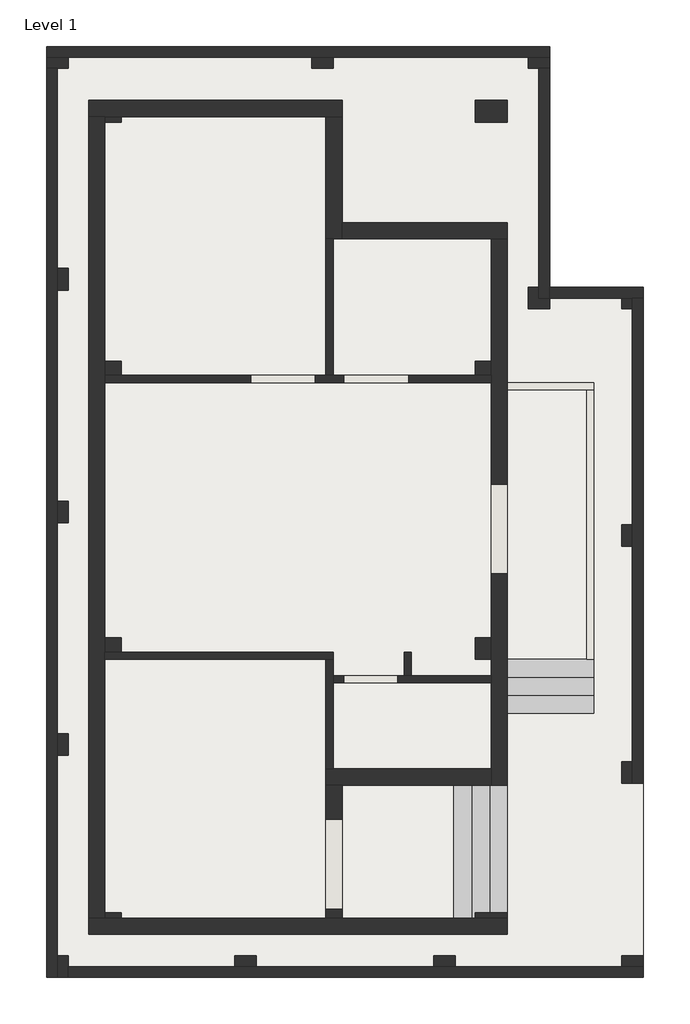
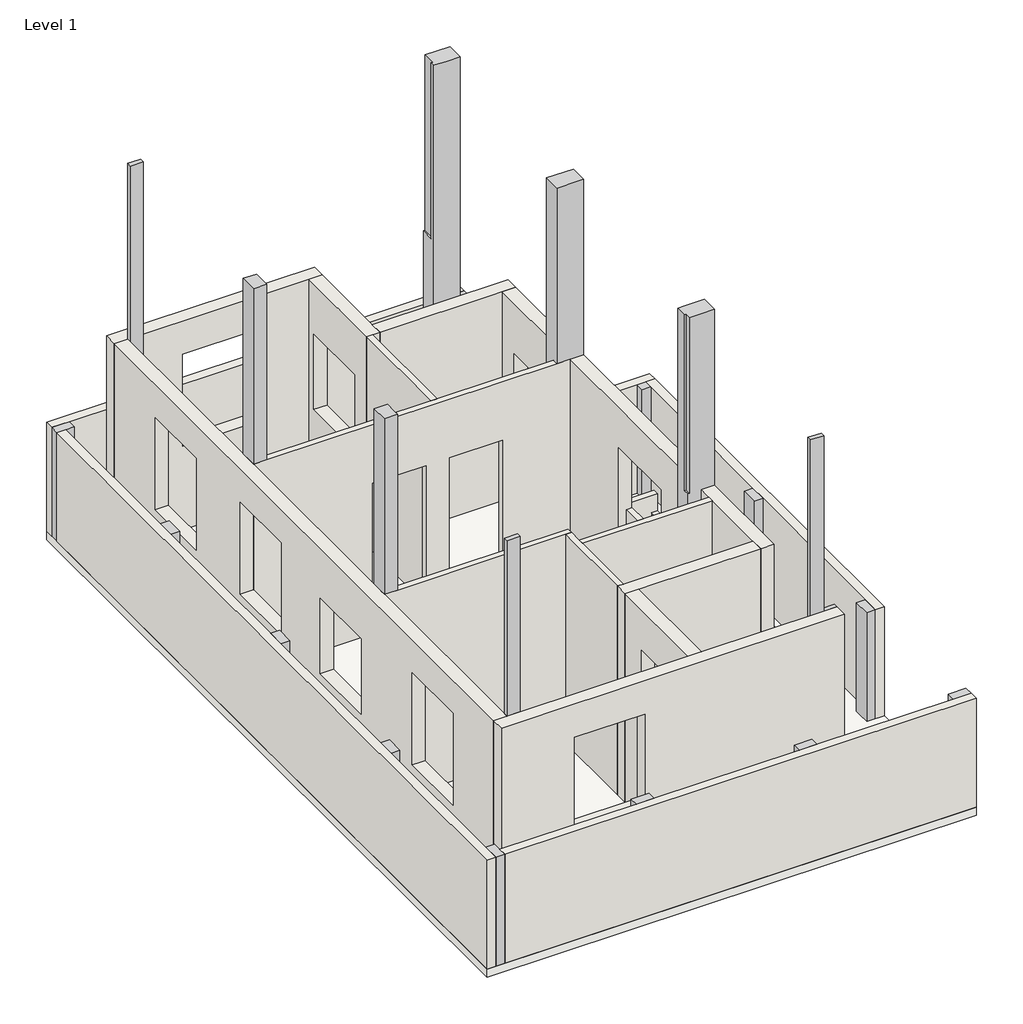
# One storey: 22 columns, 22 walls, 2 stair flights, 1 slab.
"""IFC4 building model written with IfcOpenShell, lengths in millimetres."""

from ifc_helpers import new_model, si_unit, frame, origin, origin_with_axes, place, context, project, spatial, polyline, outline, extrude, faceted_brep, element, save

model = new_model("IFC4")

# Units and contexts
model_context = context("Model", 3, world=origin())
ifc_project = project(units=[si_unit("LENGTHUNIT", "METRE", prefix="MILLI")], contexts=[model_context])

# Site, building, storey
site = spatial("IfcSite", under=ifc_project)
building = spatial("IfcBuilding", under=site)
storey = spatial("IfcBuildingStorey", under=building, Name="Level 1", Elevation=0.0)

# Columns
placement = place(None, origin())
element("IfcColumn", 1, ObjectType="Rectangular Column : 1'6\" x 1'", at=placement, inside=storey, context=model_context, shape_type="Brep", body=[
    faceted_brep([(398.6834347, -3882.8142443, 0.0), (855.8834347, -3882.8142443, 0.0), (855.8834347, -3959.0142443, 0.0), (398.6834347, -3959.0142443, 0.0), (398.6834347, -3882.8142443, 7010.4), (627.2834347, -3882.8142443, 7010.4), (627.2834347, -3882.8142443, 3810.0), (855.8834347, -3882.8142443, 3810.0), (855.8834347, -3959.0142443, 3810.0), (398.6834347, -3959.0142443, 3810.0), (398.6834347, -3959.0142443, 7010.4), (627.2834347, -3959.0142443, 7010.4), (627.2834347, -3959.0142443, 3810.0)], [[[0, 1, 2, 3]], [[1, 0, 4, 5, 6, 7]], [[2, 1, 7, 8]], [[4, 0, 3, 9, 10]], [[4, 10, 11, 5]], [[3, 2, 8, 12, 9]], [[10, 9, 12, 11]], [[12, 6, 5, 11]], [[6, 12, 8, 7]]]),
])
element("IfcColumn", 2, ObjectType="Rectangular Column : 1'6\" x 1'", at=placement, inside=storey, context=model_context, shape_type="Brep", body=[
    faceted_brep([(-4605.1165653, -3882.8142443, 0.0), (-4605.1165653, -3959.0142443, 0.0), (-4833.7165653, -3959.0142443, 0.0), (-4833.7165653, -3882.8142443, 0.0), (-4605.1165653, -3882.8142443, 7010.4), (-4833.7165653, -3882.8142443, 3810.0), (-4833.7165653, -3882.8142443, 7010.4), (-4605.1165653, -3959.0142443, 7010.4), (-4605.1165653, -3959.0142443, 3810.0), (-4833.7165653, -3959.0142443, 7010.4), (-4833.7165653, -3959.0142443, 3810.0)], [[[0, 1, 2, 3]], [[4, 0, 3, 5, 6]], [[0, 4, 7, 8, 1]], [[4, 6, 9, 7]], [[1, 8, 10, 2]], [[3, 2, 10, 5]], [[6, 5, 10, 9]], [[8, 7, 9, 10]]]),
])
element("IfcColumn", 3, ObjectType="Rectangular Column : 1'6\" x 1'", at=placement, inside=storey, context=model_context, shape_type="Brep", body=[
    faceted_brep([(-4833.7165653, 3.3857557, 0.0), (-4605.1165653, 3.3857557, 0.0), (-4605.1165653, -199.8142443, 0.0), (-4833.7165653, -199.8142443, 0.0), (-4605.1165653, 3.3857557, 7010.4), (-4833.7165653, 3.3857557, 1524.0), (-4833.7165653, 3.3857557, 2895.6), (-4833.7165653, 3.3857557, 3810.0), (-4833.7165653, 3.3857557, 7010.4), (-4605.1165653, -199.8142443, 7010.4), (-4605.1165653, -301.4142443, 7010.4), (-4605.1165653, -301.4142443, 3810.0), (-4605.1165653, -199.8142443, 3810.0), (-4833.7165653, -301.4142443, 7010.4), (-4833.7165653, -301.4142443, 3810.0), (-4833.7165653, -199.8142443, 3810.0)], [[[0, 1, 2, 3]], [[4, 1, 0, 5, 6, 7, 8]], [[1, 4, 9, 10, 11, 12, 2]], [[11, 10, 13, 14]], [[10, 9, 4, 8, 13]], [[5, 0, 3, 15, 7, 6]], [[12, 15, 3, 2]], [[15, 12, 11, 14]], [[8, 7, 15, 14, 13]]]),
])
element("IfcColumn", 4, ObjectType="Rectangular Column : 1'6\" x 1'", at=placement, inside=storey, context=model_context, shape_type="Brep", body=[
    faceted_brep([(398.6834347, -301.4142443, 0.0), (398.6834347, 3.3857557, 0.0), (627.2834347, 3.3857557, 0.0), (627.2834347, -301.4142443, 0.0), (398.6834347, 3.3857557, 7010.4), (525.6834347, 3.3857557, 7010.4), (627.2834347, 3.3857557, 7010.4), (855.8834347, 3.3857557, 7010.4), (855.8834347, 3.3857557, 3810.0), (627.2834347, 3.3857557, 3810.0), (855.8834347, -301.4142443, 7010.4), (855.8834347, -301.4142443, 3810.0), (627.2834347, -301.4142443, 3810.0), (627.2834347, -301.4142443, 7010.4), (424.0834347, -301.4142443, 7010.4), (424.0834347, -301.4142443, 3810.0), (398.6834347, -301.4142443, 3810.0), (398.6834347, -199.8142443, 3810.0), (398.6834347, -199.8142443, 7010.4), (424.0834347, -199.8142443, 7010.4), (424.0834347, -199.8142443, 3810.0)], [[[0, 1, 2, 3]], [[4, 5, 6, 7, 8, 9, 2, 1]], [[7, 10, 11, 8]], [[0, 3, 12, 11, 10, 13, 14, 15, 16]], [[1, 0, 16, 17, 18, 4]], [[7, 6, 5, 4, 18, 19, 14, 13, 10]], [[3, 2, 9, 12]], [[12, 9, 8, 11]], [[20, 19, 18, 17]], [[15, 20, 17, 16]], [[19, 20, 15, 14]]]),
])
element("IfcColumn", 5, ObjectType="Rectangular Column : 1'6\" x 1'", at=placement, inside=storey, context=model_context, shape_type="Brep", body=[
    faceted_brep([(398.6834347, 3914.9857557, 0.0), (627.2834347, 3914.9857557, 0.0), (627.2834347, 3711.7857557, 0.0), (398.6834347, 3711.7857557, 0.0), (398.6834347, 3914.9857557, 7010.4), (855.8834347, 3914.9857557, 7010.4), (855.8834347, 3914.9857557, 3810.0), (627.2834347, 3914.9857557, 3810.0), (855.8834347, 3610.1857557, 7010.4), (855.8834347, 3610.1857557, 3810.0), (627.2834347, 3610.1857557, 7010.4), (525.6834347, 3610.1857557, 7010.4), (398.6834347, 3610.1857557, 7010.4), (398.6834347, 3610.1857557, 6096.0), (398.6834347, 3610.1857557, 4724.4), (398.6834347, 3610.1857557, 3810.0), (525.6834347, 3610.1857557, 3810.0), (627.2834347, 3610.1857557, 3810.0), (398.6834347, 3711.7857557, 3810.0), (398.6834347, 3711.7857557, 7010.4), (627.2834347, 3711.7857557, 3810.0)], [[[0, 1, 2, 3]], [[4, 5, 6, 7, 1, 0]], [[5, 8, 9, 6]], [[8, 10, 11, 12, 13, 14, 15, 16, 17, 9]], [[4, 0, 3, 18, 15, 14, 13, 12, 19]], [[5, 4, 19, 12, 11, 10, 8]], [[1, 7, 20, 2]], [[7, 6, 9, 17, 20]], [[20, 18, 3, 2]], [[18, 20, 17, 16, 15]]]),
])
element("IfcColumn", 6, ObjectType="Rectangular Column : 1'6\" x 1'", at=placement, inside=storey, context=model_context, shape_type="Brep", body=[
    faceted_brep([(-4833.7165653, 3914.9857557, 0.0), (-4605.1165653, 3914.9857557, 0.0), (-4605.1165653, 3711.7857557, 0.0), (-4833.7165653, 3711.7857557, 0.0), (-4605.1165653, 3914.9857557, 7010.4), (-4833.7165653, 3914.9857557, 3810.0), (-4833.7165653, 3914.9857557, 7010.4), (-4605.1165653, 3711.7857557, 7010.4), (-4605.1165653, 3610.1857557, 7010.4), (-4605.1165653, 3610.1857557, 3810.0), (-4605.1165653, 3711.7857557, 3810.0), (-4833.7165653, 3610.1857557, 7010.4), (-4833.7165653, 3610.1857557, 3810.0), (-4833.7165653, 3711.7857557, 3810.0)], [[[0, 1, 2, 3]], [[4, 1, 0, 5, 6]], [[1, 4, 7, 8, 9, 10, 2]], [[9, 8, 11, 12]], [[8, 7, 4, 6, 11]], [[5, 0, 3, 13]], [[10, 13, 3, 2]], [[13, 10, 9, 12]], [[6, 5, 13, 12, 11]]]),
])
element("IfcColumn", 7, ObjectType="Rectangular Column : 1'6\" x 1'", at=placement, inside=storey, context=model_context, shape_type="Brep", body=[
    faceted_brep([(-4605.1165653, 7369.3857557, 0.0), (-4605.1165653, 7293.1857557, 0.0), (-4833.7165653, 7293.1857557, 0.0), (-4833.7165653, 7369.3857557, 0.0), (-4605.1165653, 7293.1857557, 7010.4), (-4605.1165653, 7369.3857557, 3810.0), (-4605.1165653, 7369.3857557, 7010.4), (-4833.7165653, 7293.1857557, 7010.4), (-4833.7165653, 7293.1857557, 3810.0), (-4833.7165653, 7369.3857557, 7010.4), (-4833.7165653, 7369.3857557, 3810.0)], [[[0, 1, 2, 3]], [[4, 1, 0, 5, 6]], [[1, 4, 7, 8, 2]], [[4, 6, 9, 7]], [[5, 0, 3, 10]], [[3, 2, 8, 10]], [[6, 5, 10, 9]], [[8, 7, 9, 10]]]),
])
element("IfcColumn", 8, ObjectType="Rectangular Column : 1'6\" x 1'", at=placement, inside=storey, context=model_context, shape_type="Brep", body=[
    faceted_brep([(398.6834347, 7597.9857557, 0.0), (855.8834347, 7597.9857557, 0.0), (855.8834347, 7293.1857557, 0.0), (398.6834347, 7293.1857557, 0.0), (398.6834347, 7597.9857557, 3810.0), (424.0834347, 7597.9857557, 3810.0), (424.0834347, 7597.9857557, 7010.4), (855.8834347, 7597.9857557, 7010.4), (855.8834347, 7293.1857557, 7010.4), (855.8834347, 7293.1857557, 3810.0), (627.2834347, 7293.1857557, 7010.4), (398.6834347, 7293.1857557, 7010.4), (398.6834347, 7369.3857557, 7010.4), (398.6834347, 7369.3857557, 3810.0), (424.0834347, 7369.3857557, 7010.4), (424.0834347, 7369.3857557, 3810.0)], [[[0, 1, 2, 3]], [[1, 0, 4, 5, 6, 7]], [[2, 1, 7, 8, 9]], [[3, 2, 9, 8, 10, 11]], [[0, 3, 11, 12, 13, 4]], [[8, 7, 6, 14, 12, 11, 10]], [[14, 15, 13, 12]], [[15, 5, 4, 13]], [[15, 14, 6, 5]]]),
])
element("IfcColumn", 9, ObjectType="Rectangular Column : 1'x1'", at=placement, inside=storey, context=model_context, shape_type="SweptSolid", body=[
    extrude(outline(polyline([(-5354.4165653, 5223.0857557), (-5354.4165653, 4918.2857557), (-5506.8165653, 4918.2857557), (-5506.8165653, 5223.0857557), (-5354.4165653, 5223.0857557)])), origin_with_axes(), (0.0, 0.0, 1.0), 1981.2),
])
element("IfcColumn", 10, ObjectType="Rectangular Column : 1'x1'", at=placement, inside=storey, context=model_context, shape_type="Brep", body=[
    faceted_brep([(-5354.4165653, 8055.1857557, 0.0), (-5506.8165653, 8055.1857557, 0.0), (-5659.2165653, 8055.1857557, 0.0), (-5659.2165653, 8207.5857557, 0.0), (-5354.4165653, 8207.5857557, 0.0), (-5354.4165653, 8055.1857557, 1981.2), (-5354.4165653, 8207.5857557, 1981.2), (-5506.8165653, 8055.1857557, 1981.2), (-5659.2165653, 8055.1857557, 1981.2), (-5659.2165653, 8207.5857557, 1981.2)], [[[0, 1, 2, 3, 4]], [[5, 0, 4, 6]], [[2, 1, 0, 5, 7, 8]], [[2, 8, 9, 3]], [[8, 7, 5, 6, 9]], [[4, 3, 9, 6]]]),
])
element("IfcColumn", 11, ObjectType="Rectangular Column : 1'x1'", at=placement, inside=storey, context=model_context, shape_type="SweptSolid", body=[
    extrude(outline(polyline([(-1607.9165653, 8055.1857557), (-1912.7165653, 8055.1857557), (-1912.7165653, 8207.5857557), (-1607.9165653, 8207.5857557), (-1607.9165653, 8055.1857557)])), origin_with_axes(), (0.0, 0.0, 1.0), 1981.2),
])
element("IfcColumn", 12, ObjectType="Rectangular Column : 1'x1'", at=placement, inside=storey, context=model_context, shape_type="Brep", body=[
    faceted_brep([(1452.7834347, 8055.1857557, 0.0), (1300.3834347, 8055.1857557, 0.0), (1147.9834347, 8055.1857557, 0.0), (1147.9834347, 8207.5857557, 0.0), (1452.7834347, 8207.5857557, 0.0), (1452.7834347, 8055.1857557, 1981.2), (1452.7834347, 8207.5857557, 1981.2), (1300.3834347, 8055.1857557, 1981.2), (1147.9834347, 8055.1857557, 1981.2), (1147.9834347, 8207.5857557, 1981.2)], [[[0, 1, 2, 3, 4]], [[5, 0, 4, 6]], [[2, 1, 0, 5, 7, 8]], [[2, 8, 9, 3]], [[8, 7, 5, 6, 9]], [[4, 3, 9, 6]]]),
])
element("IfcColumn", 13, ObjectType="Rectangular Column : 1'x1'", at=placement, inside=storey, context=model_context, shape_type="SweptSolid", body=[
    extrude(outline(polyline([(1452.7834347, 4651.5857557), (1147.9834347, 4651.5857557), (1147.9834347, 4956.3857557), (1300.3834347, 4956.3857557), (1300.3834347, 4803.9857557), (1452.7834347, 4803.9857557), (1452.7834347, 4651.5857557)])), origin_with_axes(), (0.0, 0.0, 1.0), 1981.2),
])
element("IfcColumn", 14, ObjectType="Rectangular Column : 1'x1'", at=placement, inside=storey, context=model_context, shape_type="SweptSolid", body=[
    extrude(outline(polyline([(2468.7834347, 4651.5857557), (2468.7834347, 4803.9857557), (2621.1834347, 4803.9857557), (2621.1834347, 4651.5857557), (2468.7834347, 4651.5857557)])), origin_with_axes(), (0.0, 0.0, 1.0), 1981.2),
])
element("IfcColumn", 15, ObjectType="Rectangular Column : 1'x1'", at=placement, inside=storey, context=model_context, shape_type="SweptSolid", body=[
    extrude(outline(polyline([(-5354.4165653, 1933.7857557), (-5354.4165653, 1628.9857557), (-5506.8165653, 1628.9857557), (-5506.8165653, 1933.7857557), (-5354.4165653, 1933.7857557)])), origin_with_axes(), (0.0, 0.0, 1.0), 1981.2),
])
element("IfcColumn", 16, ObjectType="Rectangular Column : 1'x1'", at=placement, inside=storey, context=model_context, shape_type="SweptSolid", body=[
    extrude(outline(polyline([(-5354.4165653, -1355.5142443), (-5354.4165653, -1660.3142443), (-5506.8165653, -1660.3142443), (-5506.8165653, -1355.5142443), (-5354.4165653, -1355.5142443)])), origin_with_axes(), (0.0, 0.0, 1.0), 1981.2),
])
element("IfcColumn", 17, ObjectType="Rectangular Column : 1'x1'", at=placement, inside=storey, context=model_context, shape_type="Brep", body=[
    faceted_brep([(-5354.4165653, -4492.4142443, 0.0), (-5354.4165653, -4644.8142443, 0.0), (-5354.4165653, -4797.2142443, 0.0), (-5506.8165653, -4797.2142443, 0.0), (-5506.8165653, -4492.4142443, 0.0), (-5354.4165653, -4492.4142443, 1981.2), (-5354.4165653, -4644.8142443, 1981.2), (-5354.4165653, -4797.2142443, 1981.2), (-5506.8165653, -4797.2142443, 1981.2), (-5506.8165653, -4492.4142443, 1981.2)], [[[0, 1, 2, 3, 4]], [[2, 1, 0, 5, 6, 7]], [[2, 7, 8, 3]], [[5, 0, 4, 9]], [[7, 6, 5, 9, 8]], [[4, 3, 8, 9]]]),
])
element("IfcColumn", 18, ObjectType="Rectangular Column : 1'x1'", at=placement, inside=storey, context=model_context, shape_type="SweptSolid", body=[
    extrude(outline(polyline([(-3000.683232, -4492.4142443), (-2695.883232, -4492.4142443), (-2695.883232, -4644.8142443), (-3000.683232, -4644.8142443), (-3000.683232, -4492.4142443)])), origin_with_axes(), (0.0, 0.0, 1.0), 1981.2),
])
element("IfcColumn", 19, ObjectType="Rectangular Column : 1'x1'", at=placement, inside=storey, context=model_context, shape_type="SweptSolid", body=[
    extrude(outline(polyline([(-189.7498986, -4492.4142443), (115.0501014, -4492.4142443), (115.0501014, -4644.8142443), (-189.7498986, -4644.8142443), (-189.7498986, -4492.4142443)])), origin_with_axes(), (0.0, 0.0, 1.0), 1981.2),
])
element("IfcColumn", 20, ObjectType="Rectangular Column : 1'x1'", at=placement, inside=storey, context=model_context, shape_type="SweptSolid", body=[
    extrude(outline(polyline([(2468.7834347, -4492.4142443), (2773.5834347, -4492.4142443), (2773.5834347, -4644.8142443), (2468.7834347, -4644.8142443), (2468.7834347, -4492.4142443)])), origin_with_axes(), (0.0, 0.0, 1.0), 1981.2),
])
element("IfcColumn", 21, ObjectType="Rectangular Column : 1'x1'", at=placement, inside=storey, context=model_context, shape_type="SweptSolid", body=[
    extrude(outline(polyline([(2468.7834347, -2054.0142443), (2468.7834347, -1749.2142443), (2621.1834347, -1749.2142443), (2621.1834347, -2054.0142443), (2468.7834347, -2054.0142443)])), origin_with_axes(), (0.0, 0.0, 1.0), 1981.2),
])
element("IfcColumn", 22, ObjectType="Rectangular Column : 1'x1'", at=placement, inside=storey, context=model_context, shape_type="SweptSolid", body=[
    extrude(outline(polyline([(2468.7834347, 1298.7857557), (2468.7834347, 1603.5857557), (2621.1834347, 1603.5857557), (2621.1834347, 1298.7857557), (2468.7834347, 1298.7857557)])), origin_with_axes(), (0.0, 0.0, 1.0), 1981.2),
])

# Slab
element("IfcSlab", 23, ObjectType="6\" floor", at=placement, inside=storey, context=model_context, shape_type="SweptSolid", body=[
    extrude(outline(polyline([(-5659.2165653, 8359.9857557), (1452.7834347, 8359.9857557), (1452.7834347, 4956.3857557), (2773.5834347, 4956.3857557), (2773.5834347, -4797.2142443), (-5659.2165653, -4797.2142443), (-5659.2165653, 8359.9857557)])), frame((0.0, 0.0, -152.4), z_axis=(0.0, 0.0, 1.0), x_axis=(1.0, 0.0, 0.0)), (0.0, 0.0, 1.0), 152.4),
])

# Stair flights
element("IfcStairFlight", 24, ObjectType="3/4\" Nosing", at=placement, inside=storey, context=model_context, shape_type="Brep", body=[
    faceted_brep([(855.8834347, -2079.4142443, 152.4), (855.8834347, -3882.8142443, 152.4), (836.8334347, -3882.8142443, 0.0), (836.8334347, -2079.4142443, 0.0), (582.8334347, -2079.4142443, 152.4), (582.8334347, -3882.8142443, 152.4), (582.8334347, -3882.8142443, 0.0), (582.8334347, -2079.4142443, 0.0), (347.8834347, -3959.0142443, 457.2), (347.8834347, -2079.4142443, 457.2), (93.8834347, -2079.4142443, 457.2), (93.8834347, -3959.0142443, 457.2), (328.8334347, -3959.0142443, 0.0), (328.8334347, -3959.0142443, 304.8), (93.8834347, -3959.0142443, 0.0), (328.8334347, -2079.4142443, 304.8), (328.8334347, -2079.4142443, 0.0), (93.8834347, -2079.4142443, 0.0), (398.6834347, -3882.8142443, 0.0), (398.6834347, -3959.0142443, 0.0), (398.6834347, -3959.0142443, 304.8), (398.6834347, -3882.8142443, 304.8), (601.8834347, -3882.8142443, 304.8), (601.8834347, -2079.4142443, 304.8)], [[[0, 1, 2, 3]], [[1, 0, 4, 5]], [[1, 5, 6, 2]], [[4, 0, 3, 7]], [[8, 9, 10, 11]], [[12, 13, 8, 11, 14]], [[15, 16, 17, 10, 9]], [[11, 10, 17, 14]], [[13, 15, 9, 8]], [[2, 6, 18, 19, 12, 14, 17, 16, 7, 3]], [[13, 20, 21, 22, 23, 15]], [[20, 13, 12, 19]], [[21, 20, 19, 18]], [[6, 5, 22, 21, 18]], [[4, 7, 16, 15, 23]], [[5, 4, 23, 22]]]),
])
element("IfcStairFlight", 25, ObjectType="3/4\" Nosing", at=placement, inside=storey, context=model_context, shape_type="Brep", body=[
    faceted_brep([(2075.0834347, -1063.4142443, 152.4), (855.8834347, -1063.4142443, 152.4), (855.8834347, -1044.3642443, 0.0), (2075.0834347, -1044.3642443, 0.0), (2075.0834347, -790.3642443, 152.4), (855.8834347, -790.3642443, 152.4), (855.8834347, -790.3642443, 0.0), (2075.0834347, -790.3642443, 0.0), (855.8834347, -809.4142443, 304.8), (2075.0834347, -809.4142443, 304.8), (2075.0834347, -536.3642443, 304.8), (855.8834347, -536.3642443, 304.8), (855.8834347, -536.3642443, 0.0), (2075.0834347, -536.3642443, 0.0), (855.8834347, -555.4142443, 457.2), (2075.0834347, -555.4142443, 457.2), (2075.0834347, -301.4142443, 457.2), (855.8834347, -301.4142443, 457.2), (855.8834347, -301.4142443, 0.0), (2075.0834347, -301.4142443, 0.0)], [[[0, 1, 2, 3]], [[1, 0, 4, 5]], [[1, 5, 6, 2]], [[4, 0, 3, 7]], [[8, 9, 10, 11]], [[6, 5, 8, 11, 12]], [[4, 7, 13, 10, 9]], [[5, 4, 9, 8]], [[14, 15, 16, 17]], [[12, 11, 14, 17, 18]], [[10, 13, 19, 16, 15]], [[17, 16, 19, 18]], [[11, 10, 15, 14]], [[2, 6, 12, 18, 19, 13, 7, 3]]]),
])

# Walls
element("IfcWall", 26, at=placement, inside=storey, context=model_context, shape_type="Brep", body=[
    faceted_brep([(-4833.7165653, 3610.1857557, 0.0), (627.2834347, 3610.1857557, 0.0), (627.2834347, 3610.1857557, 3810.0), (398.6834347, 3610.1857557, 3810.0), (-4605.1165653, 3610.1857557, 3810.0), (-4833.7165653, 3610.1857557, 3810.0), (-4833.7165653, 3610.1857557, 3200.4), (-4833.7165653, 3610.1857557, 1524.0), (-2776.3165653, 3610.1857557, 609.6), (-2776.3165653, 3610.1857557, 2743.2), (-1861.9165653, 3610.1857557, 2743.2), (-1861.9165653, 3610.1857557, 609.6), (-541.1165653, 3610.1857557, 609.6), (-1455.5165653, 3610.1857557, 609.6), (-1455.5165653, 3610.1857557, 2743.2), (-541.1165653, 3610.1857557, 2743.2), (-4833.7165653, 3711.7857557, 0.0), (-4833.7165653, 3711.7857557, 3810.0), (-4605.1165653, 3711.7857557, 3810.0), (-1709.5165653, 3711.7857557, 3810.0), (-1607.9165653, 3711.7857557, 3810.0), (398.6834347, 3711.7857557, 3810.0), (627.2834347, 3711.7857557, 3810.0), (627.2834347, 3711.7857557, 0.0), (398.6834347, 3711.7857557, 0.0), (-1607.9165653, 3711.7857557, 0.0), (-1709.5165653, 3711.7857557, 0.0), (-4605.1165653, 3711.7857557, 0.0), (-2776.3165653, 3711.7857557, 609.6), (-1861.9165653, 3711.7857557, 609.6), (-1861.9165653, 3711.7857557, 2743.2), (-2776.3165653, 3711.7857557, 2743.2), (-541.1165653, 3711.7857557, 609.6), (-541.1165653, 3711.7857557, 2743.2), (-1455.5165653, 3711.7857557, 2743.2), (-1455.5165653, 3711.7857557, 609.6)], [[[0, 1, 2, 3, 4, 5, 6, 7], [8, 9, 10, 11], [12, 13, 14, 15]], [[16, 17, 18, 19, 20, 21, 22, 23, 24, 25, 26, 27], [28, 29, 30, 31], [32, 33, 34, 35]], [[1, 0, 16, 27, 26, 25, 24, 23]], [[5, 4, 3, 2, 22, 21, 20, 19, 18, 17]], [[0, 7, 6, 5, 17, 16]], [[2, 1, 23, 22]], [[29, 28, 8, 11]], [[30, 29, 11, 10]], [[31, 30, 10, 9]], [[28, 31, 9, 8]], [[13, 12, 32, 35]], [[14, 13, 35, 34]], [[15, 14, 34, 33]], [[12, 15, 33, 32]]]),
])
element("IfcWall", 27, at=placement, inside=storey, context=model_context, shape_type="SweptSolid", body=[
    extrude(outline(polyline([(-1709.5165653, 3711.7857557), (-1709.5165653, 5642.1857557), (-1607.9165653, 5642.1857557), (-1607.9165653, 3711.7857557), (-1709.5165653, 3711.7857557)])), origin_with_axes(), (0.0, 0.0, 1.0), 3810.0),
])
element("IfcWall", 28, at=placement, inside=storey, context=model_context, shape_type="Brep", body=[
    faceted_brep([(-4833.7165653, -301.4142443, 0.0), (-1709.5165653, -301.4142443, 0.0), (-1607.9165653, -301.4142443, 0.0), (-1607.9165653, -301.4142443, 3810.0), (-1709.5165653, -301.4142443, 3810.0), (-4605.1165653, -301.4142443, 3810.0), (-4833.7165653, -301.4142443, 3810.0), (-4833.7165653, -199.8142443, 0.0), (-4833.7165653, -199.8142443, 3810.0), (-4605.1165653, -199.8142443, 3810.0), (-1607.9165653, -199.8142443, 3810.0), (-1607.9165653, -199.8142443, 0.0), (-4605.1165653, -199.8142443, 0.0)], [[[0, 1, 2, 3, 4, 5, 6]], [[7, 8, 9, 10, 11, 12]], [[2, 1, 0, 7, 12, 11]], [[6, 5, 4, 3, 10, 9, 8]], [[0, 6, 8, 7]], [[3, 2, 11, 10]]]),
])
element("IfcWall", 29, at=placement, inside=storey, context=model_context, shape_type="Brep", body=[
    faceted_brep([(-1709.5165653, -301.4142443, 0.0), (-1709.5165653, -1850.8142443, 0.0), (-1709.5165653, -1850.8142443, 3810.0), (-1709.5165653, -301.4142443, 3810.0), (-1607.9165653, -301.4142443, 0.0), (-1607.9165653, -301.4142443, 3810.0), (-1607.9165653, -530.0142443, 3810.0), (-1607.9165653, -631.6142443, 3810.0), (-1607.9165653, -1850.8142443, 3810.0), (-1607.9165653, -1850.8142443, 0.0), (-1607.9165653, -631.6142443, 0.0), (-1607.9165653, -530.0142443, 0.0)], [[[0, 1, 2, 3]], [[4, 5, 6, 7, 8, 9, 10, 11]], [[1, 0, 4, 11, 10, 9]], [[3, 2, 8, 7, 6, 5]], [[0, 3, 5, 4]], [[2, 1, 9, 8]]]),
])
element("IfcWall", 30, at=placement, inside=storey, context=model_context, shape_type="Brep", body=[
    faceted_brep([(627.2834347, -530.0142443, 0.0), (-503.6379361, -530.0142443, 0.0), (-605.2379361, -530.0142443, 0.0), (-1607.9165653, -530.0142443, 0.0), (-1607.9165653, -530.0142443, 3810.0), (-605.2379361, -530.0142443, 3810.0), (-503.6379361, -530.0142443, 3810.0), (627.2834347, -530.0142443, 3810.0), (-693.5165653, -530.0142443, 609.6), (-693.5165653, -530.0142443, 2743.2), (-1455.5165653, -530.0142443, 2743.2), (-1455.5165653, -530.0142443, 609.6), (627.2834347, -631.6142443, 0.0), (627.2834347, -631.6142443, 3810.0), (-1607.9165653, -631.6142443, 3810.0), (-1607.9165653, -631.6142443, 0.0), (-693.5165653, -631.6142443, 609.6), (-1455.5165653, -631.6142443, 609.6), (-1455.5165653, -631.6142443, 2743.2), (-693.5165653, -631.6142443, 2743.2)], [[[0, 1, 2, 3, 4, 5, 6, 7], [8, 9, 10, 11]], [[12, 13, 14, 15], [16, 17, 18, 19]], [[3, 2, 1, 0, 12, 15]], [[7, 6, 5, 4, 14, 13]], [[0, 7, 13, 12]], [[4, 3, 15, 14]], [[17, 16, 8, 11]], [[18, 17, 11, 10]], [[19, 18, 10, 9]], [[16, 19, 9, 8]]]),
])
element("IfcWall", 31, at=placement, inside=storey, context=model_context, shape_type="SweptSolid", body=[
    extrude(outline(polyline([(-503.6379361, -199.8142443), (-503.6379361, -530.0142443), (-605.2379361, -530.0142443), (-605.2379361, -199.8142443), (-503.6379361, -199.8142443)])), origin_with_axes(), (0.0, 0.0, 1.0), 3810.0),
])
element("IfcWall", 32, at=placement, inside=storey, context=model_context, shape_type="Brep", body=[
    faceted_brep([(855.8834347, 3508.5857557, 0.0), (1973.4834347, 3508.5857557, 0.0), (2075.0834347, 3508.5857557, 0.0), (2075.0834347, 3508.5857557, 609.6), (2075.0834347, 3508.5857557, 914.4), (855.8834347, 3508.5857557, 914.4), (855.8834347, 3610.1857557, 0.0), (855.8834347, 3610.1857557, 914.4), (2075.0834347, 3610.1857557, 914.4), (2075.0834347, 3610.1857557, 0.0)], [[[0, 1, 2, 3, 4, 5]], [[6, 7, 8, 9]], [[2, 1, 0, 6, 9]], [[5, 4, 8, 7]], [[0, 5, 7, 6]], [[4, 3, 2, 9, 8]]]),
])
element("IfcWall", 33, at=placement, inside=storey, context=model_context, shape_type="SweptSolid", body=[
    extrude(outline(polyline([(1973.4834347, -301.4142443), (1973.4834347, 3508.5857557), (2075.0834347, 3508.5857557), (2075.0834347, -301.4142443), (1973.4834347, -301.4142443)])), origin_with_axes(), (0.0, 0.0, 1.0), 609.6),
])
element("IfcWall", 34, ObjectType="6\" wall", at=placement, inside=storey, context=model_context, shape_type="Brep", body=[
    faceted_brep([(-5659.2165653, 8055.1857557, 0.0), (-5659.2165653, -4797.2142443, 0.0), (-5659.2165653, -4797.2142443, 1981.2), (-5659.2165653, 8055.1857557, 1981.2), (-5506.8165653, 8055.1857557, 0.0), (-5506.8165653, 8055.1857557, 1981.2), (-5506.8165653, 5223.0857557, 1981.2), (-5506.8165653, 4918.2857557, 1981.2), (-5506.8165653, 1933.7857557, 1981.2), (-5506.8165653, 1628.9857557, 1981.2), (-5506.8165653, -1355.5142443, 1981.2), (-5506.8165653, -1660.3142443, 1981.2), (-5506.8165653, -4492.4142443, 1981.2), (-5506.8165653, -4797.2142443, 1981.2), (-5506.8165653, -4797.2142443, 0.0), (-5506.8165653, -4492.4142443, 0.0), (-5506.8165653, -1660.3142443, 0.0), (-5506.8165653, -1355.5142443, 0.0), (-5506.8165653, 1628.9857557, 0.0), (-5506.8165653, 1933.7857557, 0.0), (-5506.8165653, 4918.2857557, 0.0), (-5506.8165653, 5223.0857557, 0.0)], [[[0, 1, 2, 3]], [[4, 5, 6, 7, 8, 9, 10, 11, 12, 13, 14, 15, 16, 17, 18, 19, 20, 21]], [[1, 0, 4, 21, 20, 19, 18, 17, 16, 15, 14]], [[2, 1, 14, 13]], [[3, 2, 13, 12, 11, 10, 9, 8, 7, 6, 5]], [[0, 3, 5, 4]]]),
])
element("IfcWall", 35, ObjectType="6\" wall", at=placement, inside=storey, context=model_context, shape_type="Brep", body=[
    faceted_brep([(-5354.4165653, -4797.2142443, 0.0), (2773.5834347, -4797.2142443, 0.0), (2773.5834347, -4797.2142443, 1981.2), (-5354.4165653, -4797.2142443, 1981.2), (-5354.4165653, -4644.8142443, 0.0), (-5354.4165653, -4644.8142443, 1981.2), (-3000.683232, -4644.8142443, 1981.2), (-2695.883232, -4644.8142443, 1981.2), (-189.7498986, -4644.8142443, 1981.2), (115.0501014, -4644.8142443, 1981.2), (2468.7834347, -4644.8142443, 1981.2), (2773.5834347, -4644.8142443, 1981.2), (2773.5834347, -4644.8142443, 0.0), (2468.7834347, -4644.8142443, 0.0), (115.0501014, -4644.8142443, 0.0), (-189.7498986, -4644.8142443, 0.0), (-2695.883232, -4644.8142443, 0.0), (-3000.683232, -4644.8142443, 0.0)], [[[0, 1, 2, 3]], [[4, 5, 6, 7, 8, 9, 10, 11, 12, 13, 14, 15, 16, 17]], [[1, 0, 4, 17, 16, 15, 14, 13, 12]], [[2, 1, 12, 11]], [[3, 2, 11, 10, 9, 8, 7, 6, 5]], [[0, 3, 5, 4]]]),
])
element("IfcWall", 36, ObjectType="6\" wall", at=placement, inside=storey, context=model_context, shape_type="Brep", body=[
    faceted_brep([(-5659.2165653, 8207.5857557, 0.0), (-5354.4165653, 8207.5857557, 0.0), (-1912.7165653, 8207.5857557, 0.0), (-1607.9165653, 8207.5857557, 0.0), (1147.9834347, 8207.5857557, 0.0), (1452.7834347, 8207.5857557, 0.0), (1452.7834347, 8207.5857557, 1981.2), (1147.9834347, 8207.5857557, 1981.2), (-1607.9165653, 8207.5857557, 1981.2), (-1912.7165653, 8207.5857557, 1981.2), (-5354.4165653, 8207.5857557, 1981.2), (-5659.2165653, 8207.5857557, 1981.2), (-5659.2165653, 8359.9857557, 0.0), (-5659.2165653, 8359.9857557, 1981.2), (1452.7834347, 8359.9857557, 1981.2), (1452.7834347, 8359.9857557, 0.0)], [[[0, 1, 2, 3, 4, 5, 6, 7, 8, 9, 10, 11]], [[12, 13, 14, 15]], [[5, 4, 3, 2, 1, 0, 12, 15]], [[6, 5, 15, 14]], [[11, 10, 9, 8, 7, 6, 14, 13]], [[0, 11, 13, 12]]]),
])
element("IfcWall", 37, ObjectType="6\" wall", at=placement, inside=storey, context=model_context, shape_type="Brep", body=[
    faceted_brep([(1300.3834347, 8055.1857557, 0.0), (1300.3834347, 4956.3857557, 0.0), (1300.3834347, 4803.9857557, 0.0), (1300.3834347, 4803.9857557, 1981.2), (1300.3834347, 4956.3857557, 1981.2), (1300.3834347, 8055.1857557, 1981.2), (1452.7834347, 8055.1857557, 0.0), (1452.7834347, 8055.1857557, 1981.2), (1452.7834347, 4956.3857557, 1981.2), (1452.7834347, 4803.9857557, 1981.2), (1452.7834347, 4803.9857557, 0.0), (1452.7834347, 4956.3857557, 0.0)], [[[0, 1, 2, 3, 4, 5]], [[6, 7, 8, 9, 10, 11]], [[2, 1, 0, 6, 11, 10]], [[5, 4, 3, 9, 8, 7]], [[0, 5, 7, 6]], [[3, 2, 10, 9]]]),
])
element("IfcWall", 38, ObjectType="6\" wall", at=placement, inside=storey, context=model_context, shape_type="Brep", body=[
    faceted_brep([(1452.7834347, 4803.9857557, 0.0), (2468.7834347, 4803.9857557, 0.0), (2621.1834347, 4803.9857557, 0.0), (2773.5834347, 4803.9857557, 0.0), (2773.5834347, 4803.9857557, 1981.2), (2621.1834347, 4803.9857557, 1981.2), (2468.7834347, 4803.9857557, 1981.2), (1452.7834347, 4803.9857557, 1981.2), (1452.7834347, 4956.3857557, 0.0), (1452.7834347, 4956.3857557, 1981.2), (2773.5834347, 4956.3857557, 1981.2), (2773.5834347, 4956.3857557, 0.0)], [[[0, 1, 2, 3, 4, 5, 6, 7]], [[8, 9, 10, 11]], [[3, 2, 1, 0, 8, 11]], [[7, 6, 5, 4, 10, 9]], [[0, 7, 9, 8]], [[4, 3, 11, 10]]]),
])
element("IfcWall", 39, ObjectType="6\" wall", at=placement, inside=storey, context=model_context, shape_type="Brep", body=[
    faceted_brep([(2621.1834347, 4803.9857557, 0.0), (2621.1834347, 4651.5857557, 0.0), (2621.1834347, 1603.5857557, 0.0), (2621.1834347, 1298.7857557, 0.0), (2621.1834347, -1749.2142443, 0.0), (2621.1834347, -2054.0142443, 0.0), (2621.1834347, -2054.0142443, 1981.2), (2621.1834347, -1749.2142443, 1981.2), (2621.1834347, 1298.7857557, 1981.2), (2621.1834347, 1603.5857557, 1981.2), (2621.1834347, 4651.5857557, 1981.2), (2621.1834347, 4803.9857557, 1981.2), (2773.5834347, 4803.9857557, 0.0), (2773.5834347, 4803.9857557, 1981.2), (2773.5834347, -2054.0142443, 1981.2), (2773.5834347, -2054.0142443, 0.0)], [[[0, 1, 2, 3, 4, 5, 6, 7, 8, 9, 10, 11]], [[12, 13, 14, 15]], [[5, 4, 3, 2, 1, 0, 12, 15]], [[6, 5, 15, 14]], [[11, 10, 9, 8, 7, 6, 14, 13]], [[0, 11, 13, 12]]]),
])
element("IfcWall", 40, ObjectType="9\" wall", at=placement, inside=storey, context=model_context, shape_type="Brep", body=[
    faceted_brep([(-5062.3165653, 7369.3857557, 0.0), (-4833.7165653, 7369.3857557, 0.0), (-4605.1165653, 7369.3857557, 0.0), (-1709.5165653, 7369.3857557, 0.0), (-1480.9165653, 7369.3857557, 0.0), (-1480.9165653, 7369.3857557, 3810.0), (-1709.5165653, 7369.3857557, 3810.0), (-4833.7165653, 7369.3857557, 3810.0), (-5062.3165653, 7369.3857557, 3810.0), (-3881.2165655, 7369.3857557, 1524.0), (-3881.2165655, 7369.3857557, 3200.4), (-2662.0165655, 7369.3857557, 3200.4), (-2662.0165655, 7369.3857557, 1524.0), (-1480.9165653, 7597.9857557, 0.0), (-5062.3165653, 7597.9857557, 0.0), (-5062.3165653, 7597.9857557, 3810.0), (-1480.9165653, 7597.9857557, 3810.0), (-3881.2165655, 7597.9857557, 3200.4), (-3881.2165655, 7597.9857557, 1524.0), (-2662.0165655, 7597.9857557, 1524.0), (-2662.0165655, 7597.9857557, 3200.4)], [[[0, 1, 2, 3, 4, 5, 6, 7, 8], [9, 10, 11, 12]], [[13, 14, 15, 16], [17, 18, 19, 20]], [[4, 3, 2, 1, 0, 14, 13]], [[8, 7, 6, 5, 16, 15]], [[5, 4, 13, 16]], [[0, 8, 15, 14]], [[9, 18, 17, 10]], [[10, 17, 20, 11]], [[11, 20, 19, 12]], [[18, 9, 12, 19]]]),
])
element("IfcWall", 41, ObjectType="9\" wall", at=placement, inside=storey, context=model_context, shape_type="Brep", body=[
    faceted_brep([(-1709.5165653, 7369.3857557, 0.0), (-1709.5165653, 5642.1857557, 0.0), (-1709.5165653, 5642.1857557, 3810.0), (-1709.5165653, 7369.3857557, 3810.0), (-1709.5165653, 7224.1899592, 1524.0), (-1709.5165653, 7224.1899592, 2895.6), (-1709.5165653, 6004.9899592, 2895.6), (-1709.5165653, 6004.9899592, 1524.0), (-1480.9165653, 5642.1857557, 0.0), (-1480.9165653, 5870.7857557, 0.0), (-1480.9165653, 7369.3857557, 0.0), (-1480.9165653, 7369.3857557, 3810.0), (-1480.9165653, 5870.7857557, 3810.0), (-1480.9165653, 5642.1857557, 3810.0), (-1480.9165653, 7224.1899592, 2895.6), (-1480.9165653, 7224.1899592, 1524.0), (-1480.9165653, 6004.9899592, 1524.0), (-1480.9165653, 6004.9899592, 2895.6), (-1607.9165653, 5642.1857557, 0.0), (-1607.9165653, 5642.1857557, 3810.0)], [[[0, 1, 2, 3], [4, 5, 6, 7]], [[8, 9, 10, 11, 12, 13], [14, 15, 16, 17]], [[1, 0, 10, 9, 8, 18]], [[3, 2, 19, 13, 12, 11]], [[0, 3, 11, 10]], [[2, 1, 18, 8, 13, 19]], [[4, 15, 14, 5]], [[5, 14, 17, 6]], [[6, 17, 16, 7]], [[15, 4, 7, 16]]]),
])
element("IfcWall", 42, ObjectType="9\" wall", at=placement, inside=storey, context=model_context, shape_type="Brep", body=[
    faceted_brep([(-1480.9165653, 5642.1857557, 0.0), (627.2834347, 5642.1857557, 0.0), (855.8834347, 5642.1857557, 0.0), (855.8834347, 5642.1857557, 3810.0), (627.2834347, 5642.1857557, 3810.0), (-1480.9165653, 5642.1857557, 3810.0), (-1480.9165653, 5870.7857557, 0.0), (-1480.9165653, 5870.7857557, 3810.0), (855.8834347, 5870.7857557, 3810.0), (855.8834347, 5870.7857557, 0.0)], [[[0, 1, 2, 3, 4, 5]], [[6, 7, 8, 9]], [[2, 1, 0, 6, 9]], [[5, 4, 3, 8, 7]], [[0, 5, 7, 6]], [[3, 2, 9, 8]]]),
])
element("IfcWall", 43, ObjectType="9\" wall", at=placement, inside=storey, context=model_context, shape_type="Brep", body=[
    faceted_brep([(627.2834347, 5642.1857557, 0.0), (627.2834347, 3914.9857557, 0.0), (627.2834347, 3711.7857557, 0.0), (627.2834347, 3610.1857557, 0.0), (627.2834347, 3.3857557, 0.0), (627.2834347, -301.4142443, 0.0), (627.2834347, -530.0142443, 0.0), (627.2834347, -631.6142443, 0.0), (627.2834347, -1850.8142443, 0.0), (627.2834347, -2079.4142443, 0.0), (627.2834347, -2079.4142443, 3810.0), (627.2834347, -1850.8142443, 3810.0), (627.2834347, -631.6142443, 3810.0), (627.2834347, -530.0142443, 3810.0), (627.2834347, -301.4142443, 3810.0), (627.2834347, 3.3857557, 3810.0), (627.2834347, 3610.1857557, 3810.0), (627.2834347, 3711.7857557, 3810.0), (627.2834347, 3914.9857557, 3810.0), (627.2834347, 5642.1857557, 3810.0), (627.2834347, 2175.0857557, 609.6), (627.2834347, 2175.0857557, 3073.4), (627.2834347, 905.0857557, 3073.4), (627.2834347, 905.0857557, 609.6), (627.2834347, 5286.5857559, 1524.0), (627.2834347, 5286.5857559, 2895.6), (627.2834347, 4067.3857559, 2895.6), (627.2834347, 4067.3857559, 1524.0), (627.2834347, -968.1642443, 2895.6), (627.2834347, -1577.7642443, 2895.6), (627.2834347, -1577.7642443, 2286.0), (627.2834347, -968.1642443, 2286.0), (855.8834347, -2079.4142443, 0.0), (855.8834347, 3508.5857557, 0.0), (855.8834347, 3610.1857557, 0.0), (855.8834347, 5642.1857557, 0.0), (855.8834347, 5642.1857557, 3810.0), (855.8834347, 3914.9857557, 3810.0), (855.8834347, 3610.1857557, 3810.0), (855.8834347, 3.3857557, 3810.0), (855.8834347, -301.4142443, 3810.0), (855.8834347, -2079.4142443, 3810.0), (855.8834347, 2175.0857557, 609.6), (855.8834347, 905.0857557, 609.6), (855.8834347, 905.0857557, 3073.4), (855.8834347, 2175.0857557, 3073.4), (855.8834347, 5286.5857559, 2895.6), (855.8834347, 5286.5857559, 1524.0), (855.8834347, 4067.3857559, 1524.0), (855.8834347, 4067.3857559, 2895.6), (855.8834347, -968.1642443, 2895.6), (855.8834347, -968.1642443, 2286.0), (855.8834347, -1577.7642443, 2286.0), (855.8834347, -1577.7642443, 2895.6)], [[[0, 1, 2, 3, 4, 5, 6, 7, 8, 9, 10, 11, 12, 13, 14, 15, 16, 17, 18, 19], [20, 21, 22, 23], [24, 25, 26, 27], [28, 29, 30, 31]], [[32, 33, 34, 35, 36, 37, 38, 39, 40, 41], [42, 43, 44, 45], [46, 47, 48, 49], [50, 51, 52, 53]], [[9, 8, 7, 6, 5, 4, 3, 2, 1, 0, 35, 34, 33, 32]], [[19, 18, 17, 16, 15, 14, 13, 12, 11, 10, 41, 40, 39, 38, 37, 36]], [[0, 19, 36, 35]], [[10, 9, 32, 41]], [[21, 20, 42, 45]], [[22, 21, 45, 44]], [[23, 22, 44, 43]], [[20, 23, 43, 42]], [[24, 47, 46, 25]], [[25, 46, 49, 26]], [[26, 49, 48, 27]], [[47, 24, 27, 48]], [[51, 50, 28, 31]], [[52, 51, 31, 30]], [[53, 52, 30, 29]], [[50, 53, 29, 28]]]),
])
element("IfcWall", 44, ObjectType="9\" wall", at=placement, inside=storey, context=model_context, shape_type="Brep", body=[
    faceted_brep([(627.2834347, -1850.8142443, 0.0), (-1607.9165653, -1850.8142443, 0.0), (-1709.5165653, -1850.8142443, 0.0), (-1709.5165653, -1850.8142443, 3810.0), (-1607.9165653, -1850.8142443, 3810.0), (627.2834347, -1850.8142443, 3810.0), (627.2834347, -2079.4142443, 0.0), (627.2834347, -2079.4142443, 3810.0), (-1480.9165653, -2079.4142443, 3810.0), (-1709.5165653, -2079.4142443, 3810.0), (-1709.5165653, -2079.4142443, 0.0), (-1480.9165653, -2079.4142443, 0.0)], [[[0, 1, 2, 3, 4, 5]], [[6, 7, 8, 9, 10, 11]], [[2, 1, 0, 6, 11, 10]], [[5, 4, 3, 9, 8, 7]], [[0, 5, 7, 6]], [[3, 2, 10, 9]]]),
])
element("IfcWall", 45, ObjectType="9\" wall", at=placement, inside=storey, context=model_context, shape_type="SweptSolid", body=[
    extrude(outline(polyline([(-2079.4142443, 0.0), (-3959.0142443, 0.0), (-3959.0142443, 3810.0), (-2079.4142443, 3810.0), (-2079.4142443, 0.0)]), holes=[polyline([(-2562.0098448, 609.6), (-2562.0098448, 3073.4), (-3832.0098448, 3073.4), (-3832.0098448, 609.6), (-2562.0098448, 609.6)])]), frame((-1709.5165653, 0.0, 0.0), z_axis=(1.0, 0.0, 0.0), x_axis=(0.0, 1.0, 0.0)), (0.0, 0.0, 1.0), 228.6),
])
element("IfcWall", 46, ObjectType="9\" wall", at=placement, inside=storey, context=model_context, shape_type="Brep", body=[
    faceted_brep([(855.8834347, -3959.0142443, 0.0), (398.6834347, -3959.0142443, 0.0), (-1480.9165653, -3959.0142443, 0.0), (-1709.5165653, -3959.0142443, 0.0), (-4605.1165653, -3959.0142443, 0.0), (-4833.7165653, -3959.0142443, 0.0), (-5062.3165653, -3959.0142443, 0.0), (-5062.3165653, -3959.0142443, 3810.0), (-4833.7165653, -3959.0142443, 3810.0), (-1709.5165653, -3959.0142443, 3810.0), (-1480.9165653, -3959.0142443, 3810.0), (627.2834347, -3959.0142443, 3810.0), (855.8834347, -3959.0142443, 3810.0), (-3804.1534291, -3959.0142443, 3200.4), (-3804.1534291, -3959.0142443, 1524.0), (-2584.9534291, -3959.0142443, 1524.0), (-2584.9534291, -3959.0142443, 3200.4), (-5062.3165653, -4187.6142443, 0.0), (855.8834347, -4187.6142443, 0.0), (855.8834347, -4187.6142443, 3810.0), (-5062.3165653, -4187.6142443, 3810.0), (-3804.1534291, -4187.6142443, 1524.0), (-3804.1534291, -4187.6142443, 3200.4), (-2584.9534291, -4187.6142443, 3200.4), (-2584.9534291, -4187.6142443, 1524.0)], [[[0, 1, 2, 3, 4, 5, 6, 7, 8, 9, 10, 11, 12], [13, 14, 15, 16]], [[17, 18, 19, 20], [21, 22, 23, 24]], [[6, 5, 4, 3, 2, 1, 0, 18, 17]], [[12, 11, 10, 9, 8, 7, 20, 19]], [[0, 12, 19, 18]], [[7, 6, 17, 20]], [[21, 14, 13, 22]], [[22, 13, 16, 23]], [[23, 16, 15, 24]], [[14, 21, 24, 15]]]),
])
element("IfcWall", 47, ObjectType="9\" wall", at=placement, inside=storey, context=model_context, shape_type="Brep", body=[
    faceted_brep([(-4833.7165653, -3959.0142443, 0.0), (-4833.7165653, -3882.8142443, 0.0), (-4833.7165653, -301.4142443, 0.0), (-4833.7165653, -199.8142443, 0.0), (-4833.7165653, 3.3857557, 0.0), (-4833.7165653, 3610.1857557, 0.0), (-4833.7165653, 3711.7857557, 0.0), (-4833.7165653, 3914.9857557, 0.0), (-4833.7165653, 7293.1857557, 0.0), (-4833.7165653, 7369.3857557, 0.0), (-4833.7165653, 7369.3857557, 3810.0), (-4833.7165653, 3711.7857557, 3810.0), (-4833.7165653, 3610.1857557, 3810.0), (-4833.7165653, -199.8142443, 3810.0), (-4833.7165653, -301.4142443, 3810.0), (-4833.7165653, -3959.0142443, 3810.0), (-4833.7165653, 3610.1857557, 3200.4), (-4833.7165653, 3610.1857557, 1524.0), (-4833.7165653, 2390.9857558, 1524.0), (-4833.7165653, 2390.9857558, 3200.4), (-4833.7165653, 6150.1857559, 3200.4), (-4833.7165653, 6150.1857559, 1524.0), (-4833.7165653, 4930.9857559, 1524.0), (-4833.7165653, 4930.9857559, 3200.4), (-4833.7165653, -1520.6142441, 3200.4), (-4833.7165653, -1520.6142441, 1524.0), (-4833.7165653, -2739.8142441, 1524.0), (-4833.7165653, -2739.8142441, 3200.4), (-4833.7165653, 3.3857557, 1524.0), (-4833.7165653, 3.3857557, 2895.6), (-4833.7165653, 1222.5857557, 2895.6), (-4833.7165653, 1222.5857557, 1524.0), (-5062.3165653, 7369.3857557, 0.0), (-5062.3165653, -3959.0142443, 0.0), (-5062.3165653, -3959.0142443, 3810.0), (-5062.3165653, 7369.3857557, 3810.0), (-5062.3165653, 3610.1857557, 1524.0), (-5062.3165653, 3610.1857557, 3200.4), (-5062.3165653, 2390.9857558, 3200.4), (-5062.3165653, 2390.9857558, 1524.0), (-5062.3165653, 6150.1857559, 1524.0), (-5062.3165653, 6150.1857559, 3200.4), (-5062.3165653, 4930.9857559, 3200.4), (-5062.3165653, 4930.9857559, 1524.0), (-5062.3165653, -1520.6142441, 1524.0), (-5062.3165653, -1520.6142441, 3200.4), (-5062.3165653, -2739.8142441, 3200.4), (-5062.3165653, -2739.8142441, 1524.0), (-5062.3165653, 3.3857557, 2895.6), (-5062.3165653, 3.3857557, 1524.0), (-5062.3165653, 1222.5857557, 1524.0), (-5062.3165653, 1222.5857557, 2895.6)], [[[0, 1, 2, 3, 4, 5, 6, 7, 8, 9, 10, 11, 12, 13, 14, 15], [16, 17, 18, 19], [20, 21, 22, 23], [24, 25, 26, 27], [28, 29, 30, 31]], [[32, 33, 34, 35], [36, 37, 38, 39], [40, 41, 42, 43], [44, 45, 46, 47], [48, 49, 50, 51]], [[9, 8, 7, 6, 5, 4, 3, 2, 1, 0, 33, 32]], [[15, 14, 13, 12, 11, 10, 35, 34]], [[10, 9, 32, 35]], [[0, 15, 34, 33]], [[36, 17, 16, 37]], [[37, 16, 19, 38]], [[38, 19, 18, 39]], [[17, 36, 39, 18]], [[20, 41, 40, 21]], [[41, 20, 23, 42]], [[42, 23, 22, 43]], [[21, 40, 43, 22]], [[24, 45, 44, 25]], [[45, 24, 27, 46]], [[46, 27, 26, 47]], [[25, 44, 47, 26]], [[48, 29, 28, 49]], [[29, 48, 51, 30]], [[30, 51, 50, 31]], [[49, 28, 31, 50]]]),
])

save(model, "model.ifc")

# Revit data of these elements
# Type "Rectangular Column : 1'6\" x 1'"
#   Assembly Code = "B1010200"
#   Depth = 1' - 6"
#   Offset Base = 0' - 0"
#   Offset Top = 0' - 0"
#   Width = 1' - 0"
#   Material = none
# Type "Rectangular Column : 1'x1'"
#   Assembly Code = "B1010200"
#   Depth = 1' - 0"
#   Offset Base = 0' - 0"
#   Offset Top = 0' - 0"
#   Width = 1' - 0"
#   Material = none
# Type "6\" floor"
#   Assembly Code = "B1010"
#   Function = 0
#   Layers, outside or top first: 0' - 6" no material (function 1)
# Type
#   Assembly Code = "B2010"
#   Layers, outside or top first: 0' - 4" "01-9\" wall" (function 1)
# Type "6\" wall"
#   Assembly Code = "B2010"
#   Layers, outside or top first: 0' - 6" no material (function 1)
# Type "9\" wall"
#   Assembly Code = "B2010"
#   Layers, outside or top first: 0' - 9" "01-9\" wall" (function 1)
# Elements 1, 2, 3, 4, 5, 6, 7, 8 (IfcColumn, "Rectangular Column : 1'6\" x 1'")
#   Phase Created = New Construction
#   Materials on its faces: "01-9\" wall"
# Elements 9, 10, 11, 12, 13, 14, 15, 16, 17, 18, 19, 20, 21, 22 (IfcColumn, "Rectangular Column : 1'x1'")
#   Phase Created = New Construction
#   Materials on its faces: "Default Wall"
# Element 23 (IfcSlab, "6\" floor")
#   built-in parameter 1001955 = 3.14159 (stored number, unit not read)
#   Height Offset From Level = 0' - 0"
#   Phase Created = New Construction
#   Materials on its faces: "Default Floor"
# Elements 24, 25 (IfcStairFlight, "3/4\" Nosing")
#   Phase Created = New Construction
#   Materials on its faces: "Concrete, Cast-in-Place gray"
# Elements 26, 27, 28, 29, 30, 31 (IfcWall)
#   Top Offset = 0' - 0"
#   Base Offset = 0' - 0"
#   wall height = 12' - 6"
#   Phase Created = New Construction
#   Base Constraint = Level 1
#   Top Constraint = Level 3
#   Materials on its faces: "01-9\" wall"
# Element 32 (IfcWall)
#   Top Offset = 1' - 0"
#   Base Offset = 0' - 0"
#   wall height = 3' - 0"
#   Phase Created = New Construction
#   Base Constraint = Level 1
#   Top Constraint = Level 2
#   Materials on its faces: "01-9\" wall"
# Element 33 (IfcWall)
#   Top Offset = 0' - 0"
#   Base Offset = 0' - 0"
#   wall height = 2' - 0"
#   Phase Created = New Construction
#   Base Constraint = Level 1
#   Top Constraint = Level 2
#   Materials on its faces: "01-9\" wall"
# Elements 34, 35, 36, 37, 38, 39 (IfcWall, "6\" wall")
#   Top Offset = -6' - 0"
#   Base Offset = 0' - 0"
#   wall height = 6' - 6"
#   Phase Created = New Construction
#   Base Constraint = Level 1
#   Top Constraint = Level 3
#   Materials on its faces: "Default Wall"
# Elements 40, 41, 42, 43, 44, 45, 46, 47 (IfcWall, "9\" wall")
#   Top Offset = 0' - 0"
#   Base Offset = 0' - 0"
#   wall height = 12' - 6"
#   Phase Created = New Construction
#   Base Constraint = Level 1
#   Top Constraint = Level 3
#   Materials on its faces: "01-9\" wall"
# Materials
#   "01-9\" wall": class "Generic", colour RGB 244 244 244, transparency 0, Cost = 0
#   "Default Wall": colour RGB 128 128 128, transparency 0, Cost = 0
#   "Default Floor": colour RGB 128 128 128, transparency 0, Cost = 0
#   "Concrete, Cast-in-Place gray": class "Concrete", colour RGB 192 192 192, transparency 0, Description = "Cast-in-place concrete", Cost = 0
